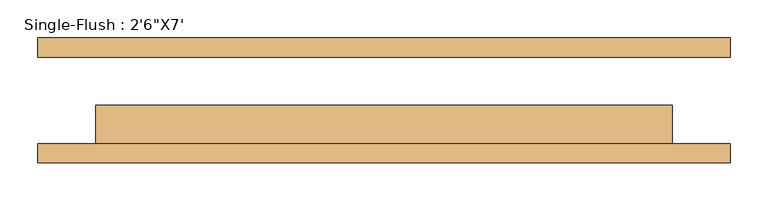
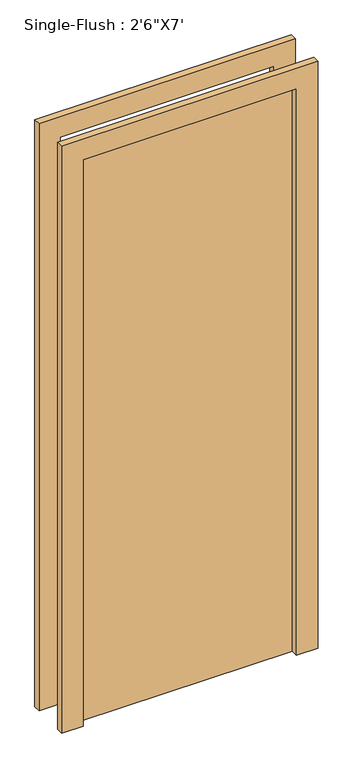
"""IFC4 building model written with IfcOpenShell, lengths in millimetres: door geometry."""

from ifc_helpers import new_model, si_unit, frame, origin, origin_with_axes, place, context, project, spatial, polyline, outline, extrude, source, transform, mapped, element, save


def door_78caadf7(model_context):
    return source(origin(), model_context, "Body", "SweptSolid", [
        extrude(outline(polyline([(2209.8, -457.2), (0.0, -457.2), (0.0, -381.0), (2133.6, -381.0), (2133.6, 381.0), (0.0, 381.0), (0.0, 457.2), (2209.8, 457.2), (2209.8, -457.2)])), frame((0.0, -82.55, 0.0), z_axis=(0.0, 1.0, 0.0), x_axis=(0.0, 0.0, 1.0)), (0.0, 0.0, 1.0), 25.4),
        extrude(outline(polyline([(2209.8, 457.2), (2209.8, -457.2), (0.0, -457.2), (0.0, -381.0), (2133.6, -381.0), (2133.6, 381.0), (0.0, 381.0), (0.0, 457.2), (2209.8, 457.2)])), frame((0.0, 57.15, 0.0), z_axis=(0.0, 1.0, 0.0), x_axis=(0.0, 0.0, 1.0)), (0.0, 0.0, 1.0), 25.4),
        extrude(outline(polyline([(381.0, -6.35), (381.0, -57.15), (-381.0, -57.15), (-381.0, -6.35), (381.0, -6.35)])), origin_with_axes(), (0.0, 0.0, 1.0), 2133.6),
    ])


if __name__ == "__main__":
    model = new_model("IFC4")
    model_context = context("Model", 3, world=origin())
    ifc_project = project(units=[si_unit("LENGTHUNIT", "METRE", prefix="MILLI")], contexts=[model_context])
    site = spatial("IfcSite", under=ifc_project)
    building = spatial("IfcBuilding", under=site)
    placement = place(None, origin())
    door_shape = door_78caadf7(model_context)
    element("IfcDoor", 1, ObjectType="Single-Flush : 2'6\"X7'", at=placement, inside=building, context=model_context, shape_type="MappedRepresentation", body=[
        mapped(door_shape, transform((0.0, 0.0, 0.0), x_axis=(1.0, 0.0, 0.0), y_axis=(0.0, 1.0, 0.0), z_axis=(0.0, 0.0, 1.0))),
    ])
    save(model, "model.ifc")

# Revit data of these elements
# Type "Single-Flush : 2'6\"X7'"
#   Type Mark = "9"
#   Construction Type Id = "MDOOR"
#   Assembly Code = "C1020"
#   Analytic Construction = "Metal"
#   Thickness = 0' - 2"
#   Heat Transfer Coefficient (U) = 0.651978 BTU/(h·ft²·°F)
#   Height = 7' - 0"
#   Trim Projection Ext = 0' - 1"
#   Trim Projection Int = 0' - 1"
#   Trim Width = 0' - 3"
#   Width = 2' - 6"
#   Define Thermal Properties by = 1
#   Door Material = Door - Panel
#   Frame Material = Door - Frame
#   Visual Light Transmittance = 0
#   Solar Heat Gain Coefficient = 0
#   Function = (empty or 0)
#   Wall Closure = (empty or 0)
# Element 1 (IfcDoor, "Single-Flush : 2'6\"X7'")
#   Materials on its faces: "Door - Frame", "Door - Panel"
# Materials
#   "Door - Panel": class "Wood", colour RGB 210 159 95, transparency 0, Cost = 0
#   "Door - Frame": colour RGB 118 70 51, transparency 0, Cost = 0
